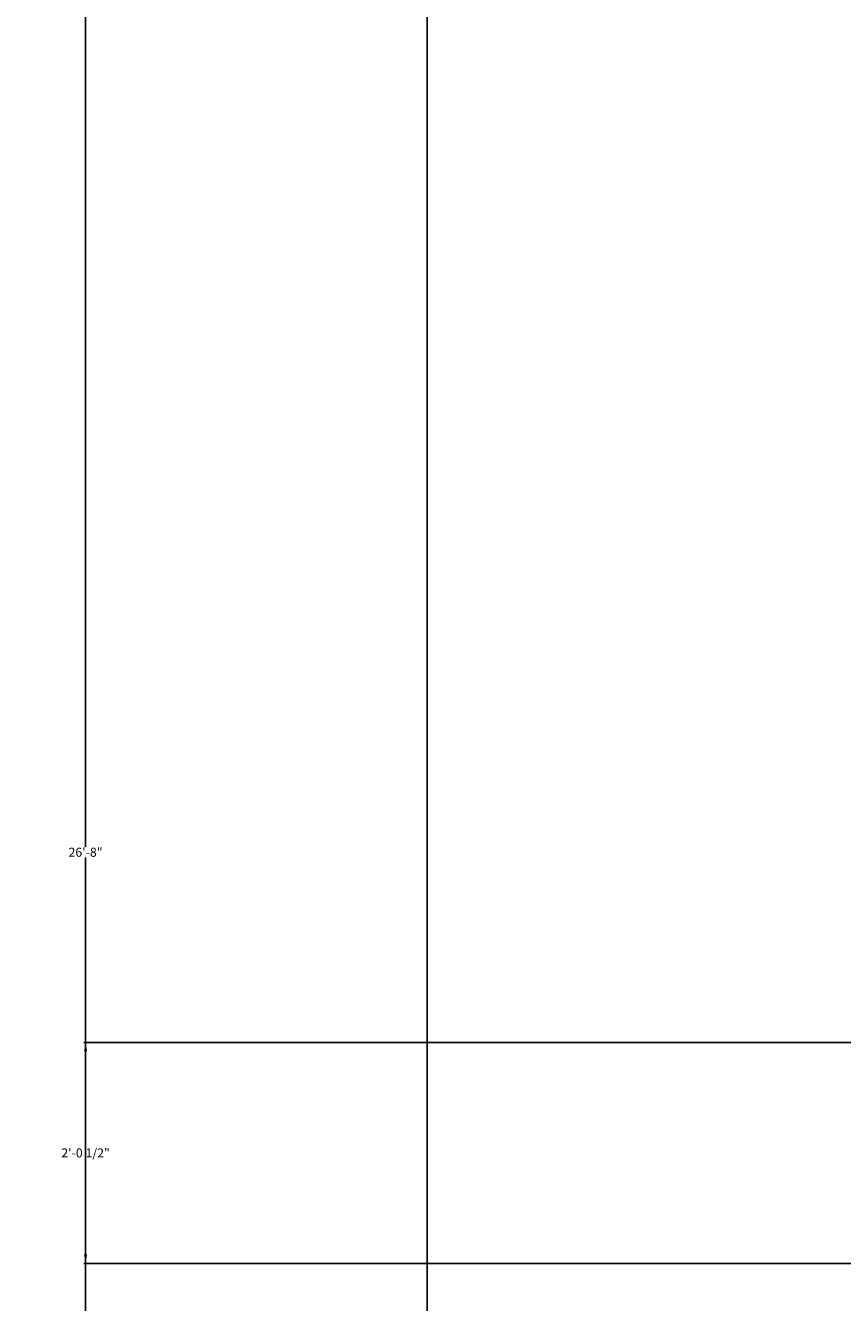
# Model space of a CAD drawing. Units: inches. Extents: x -304 to 580, y 363 to 1149.
# Tile 3 of 11: x -115 to -25, y 512 to 653. Entities that reach past the tile are written whole.
import ezdxf

# ---------------------------------------------------------------- set-up
doc = ezdxf.new("R2010")
doc.units = ezdxf.units.IN
doc.header["$MEASUREMENT"] = 0
doc.layers.add('A-ANNO-DIMS', color=2, linetype='Continuous', lineweight=13)
doc.layers.add('A-FLOR-OTLN', color=2, linetype='Continuous', lineweight=25)
doc.styles.get("Standard").update_dxf_attribs({"font": 'arial.ttf'})
doc.dimstyles.get("Standard").update_dxf_attribs({"dimtxt": 1, "dimasz": 1, "dimexe": 0.18, "dimexo": 0.0625, "dimgap": 0.09, "dimtad": 0, "dimtih": 1, "dimtoh": 1, "dimdec": 0, "dimzin": 0, "dimdsep": 46, "dimlunit": 3, "dimtxsty": 'Standard', "dimcen": 0.09, "dimadec": 0, "dimazin": 0, "dimtfac": 1, "dimtdec": 0, "dimtofl": 0, "dimtmove": 0, "dimatfit": 3, "dimfxl": 1, "dimtolj": 1, "dimtzin": 0, "dimarcsym": 0})

# ---------------------------------------------------------------- blocks, each defined once
blk = doc.blocks.new('*D1')
at = {"layer": 'A-ANNO-DIMS', "color": 0, "lineweight": -2, "transparency": 16777216}
for p, q in [((-22.63, 1004.95), (-237.62, 1004.95)), ((-237.44, 1003.95), (-237.44, 721.93)), ((-237.44, 402.95), (-237.44, 684.96)), ((-22.63, 401.95), (-237.62, 401.95))]:
    blk.add_line(p, q, dxfattribs=at)
at = {"layer": 'A-ANNO-DIMS', "color": 0, "transparency": 16777216}
for points in [[(-237.61, 1003.95), (-237.28, 1003.95), (-237.44, 1004.95)], [(-237.61, 402.95), (-237.28, 402.95), (-237.44, 401.95)]]:
    blk.add_solid(points, dxfattribs=at)
at = {"layer": 'Defpoints', "color": 0, "transparency": 16777216}
for p in [(-22.57, 1004.95), (-237.44, 401.95), (-22.57, 401.95)]:
    blk.add_point(p, dxfattribs=at)
at = {"layer": 'A-ANNO-DIMS', "color": 0, "transparency": 16777216, "insert": (-237.44, 703.45), "char_height": 1, "attachment_point": 5}
blk.add_mtext('\\A1;{\\H36x;50\'-3"}', dxfattribs=at)
blk = doc.blocks.new('*D30')
at = {"layer": 'A-ANNO-DIMS', "color": 0, "lineweight": -2, "transparency": 16777216}
for p, q in [((-70.63, 721.98), (-108.5, 721.98)), ((-108.32, 720.98), (-108.32, 562.56)), ((-108.32, 402.95), (-108.32, 561.36)), ((-70.63, 401.95), (-108.5, 401.95))]:
    blk.add_line(p, q, dxfattribs=at)
at = {"layer": 'A-ANNO-DIMS', "color": 0, "transparency": 16777216}
for points in [[(-108.49, 720.98), (-108.15, 720.98), (-108.32, 721.98)], [(-108.49, 402.95), (-108.15, 402.95), (-108.32, 401.95)]]:
    blk.add_solid(points, dxfattribs=at)
at = {"layer": 'Defpoints', "color": 0, "transparency": 16777216}
for p in [(-108.32, 721.98), (-70.57, 721.98), (-70.57, 401.95)]:
    blk.add_point(p, dxfattribs=at)
at = {"layer": 'A-ANNO-DIMS', "color": 0, "transparency": 16777216, "insert": (-108.32, 561.96), "char_height": 1, "attachment_point": 5}
blk.add_mtext('\\A1;26\'-8"', dxfattribs=at)
blk = doc.blocks.new('*D37')
at = {"layer": 'A-ANNO-DIMS', "color": 0, "lineweight": -2, "transparency": 16777216}
for p, q in [((-22.63, 540.95), (-108.5, 540.95)), ((-108.32, 539.95), (-108.32, 529.34)), ((-108.32, 517.51), (-108.32, 528.12)), ((-22.63, 516.51), (-108.5, 516.51))]:
    blk.add_line(p, q, dxfattribs=at)
at = {"layer": 'A-ANNO-DIMS', "color": 0, "transparency": 16777216}
for points in [[(-108.49, 539.95), (-108.15, 539.95), (-108.32, 540.95)], [(-108.49, 517.51), (-108.15, 517.51), (-108.32, 516.51)]]:
    blk.add_solid(points, dxfattribs=at)
at = {"layer": 'Defpoints', "color": 0, "transparency": 16777216}
for p in [(-108.32, 540.95), (-22.57, 540.95), (-22.57, 516.51)]:
    blk.add_point(p, dxfattribs=at)
at = {"layer": 'A-ANNO-DIMS', "color": 0, "transparency": 16777216, "insert": (-108.32, 528.73), "char_height": 1, "attachment_point": 5}
blk.add_mtext('\\A1;2\'-0 1/2"', dxfattribs=at)

msp = doc.modelspace()

# ---------------------------------------------------------------- linework, layer by layer
at = {"layer": 'A-FLOR-OTLN'}
msp.add_line((-70.57, 721.98), (-70.57, 401.95), dxfattribs=at)

# ---------------------------------------------------------------- dimensions: what is measured, and where the dimension line sits
at = {"layer": 'A-ANNO-DIMS'}
dim = msp.add_linear_dim(base=(-237.44, 401.95), p1=(-22.57, 1004.95), p2=(-22.57, 401.95), angle=90, text='{\\H36x;<>}', dimstyle='Standard', override={"dimclrd": 0, "dimclre": 0, "dimclrt": 0}, dxfattribs=at)
dim.commit()
dim.dimension.update_dxf_attribs({"geometry": '*D1', "text_midpoint": (-237.44, 703.45)})
for base, p1, p2, picture, middle in [((-108.32, 721.98), (-70.57, 401.95), (-70.57, 721.98), '*D30', (-108.32, 561.96)), ((-108.32, 540.95), (-22.57, 516.51), (-22.57, 540.95), '*D37', (-108.32, 528.73))]:
    dim = msp.add_linear_dim(base=base, p1=p1, p2=p2, angle=90, dimstyle='Standard', override={"dimdec": 1, "dimlfac": 1, "dimrnd": 0, "dimzin": 1, "dimdsep": 46, "dimlunit": 4, "dimfrac": 2}, dxfattribs=at)
    dim.commit()
    dim.dimension.update_dxf_attribs({"geometry": picture, "text_midpoint": middle})

doc.saveas('drawing.dxf')
